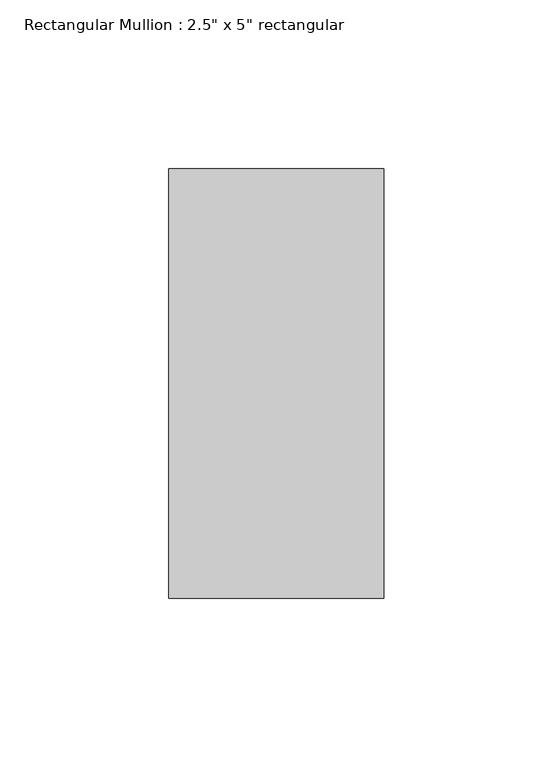
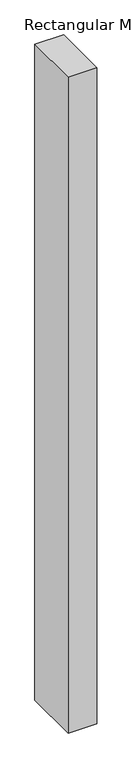
"""IFC4 building model written with IfcOpenShell, lengths in millimetres: member geometry."""

from ifc_helpers import new_model, si_unit, frame, origin, place, context, project, spatial, polyline, outline, extrude, source, transform, mapped, element, save


def member_29542bbd(model_context):
    return source(origin(), model_context, "Body", "SweptSolid", [
        extrude(outline(polyline([(0.0, 63.5), (0.0, -63.5), (-63.5, -63.5), (-63.5, 63.5), (0.0, 63.5)])), frame((0.0, 0.0, -1528.6649662), z_axis=(0.0, 0.0, 1.0), x_axis=(1.0, 0.0, 0.0)), (0.0, 0.0, 1.0), 1528.6649662),
    ])


if __name__ == "__main__":
    model = new_model("IFC4")
    model_context = context("Model", 3, world=origin())
    ifc_project = project(units=[si_unit("LENGTHUNIT", "METRE", prefix="MILLI")], contexts=[model_context])
    site = spatial("IfcSite", under=ifc_project)
    building = spatial("IfcBuilding", under=site)
    placement = place(None, origin())
    member_shape = member_29542bbd(model_context)
    element("IfcMember", 1, ObjectType="Rectangular Mullion : 2.5\" x 5\" rectangular", at=placement, inside=building, context=model_context, shape_type="MappedRepresentation", body=[
        mapped(member_shape, transform((0.0, 0.0, 0.0), x_axis=(1.0, 0.0, 0.0), y_axis=(0.0, 1.0, 0.0), z_axis=(0.0, 0.0, 1.0))),
    ])
    save(model, "model.ifc")

# Revit data of these elements
# Type "Rectangular Mullion : 2.5\" x 5\" rectangular"
#   built-in parameter 1007304 = 0.416667 (stored number, unit not read)
#   built-in parameter 1007301 = 0.104167 (stored number, unit not read)
#   built-in parameter 1007300 = 0.104167 (stored number, unit not read)
# Element 1 (IfcMember, "Rectangular Mullion : 2.5\" x 5\" rectangular")
#   Materials on its faces: "Aluminum"
# Materials
#   "Aluminum": class "Metal", colour RGB 247 247 247, transparency 0, Description = "Aluminum 6061", Cost = 0
